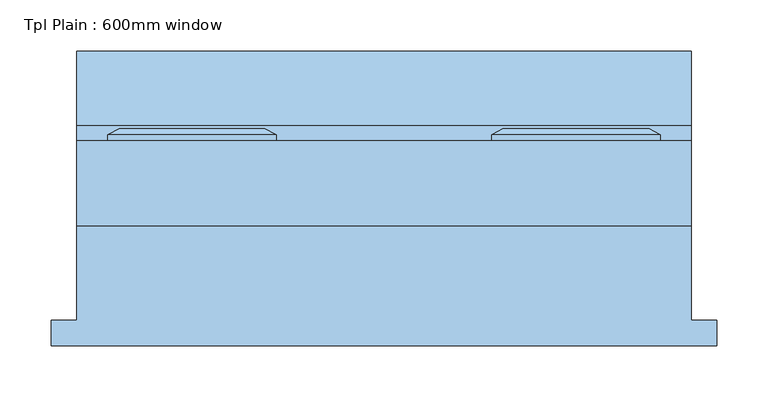
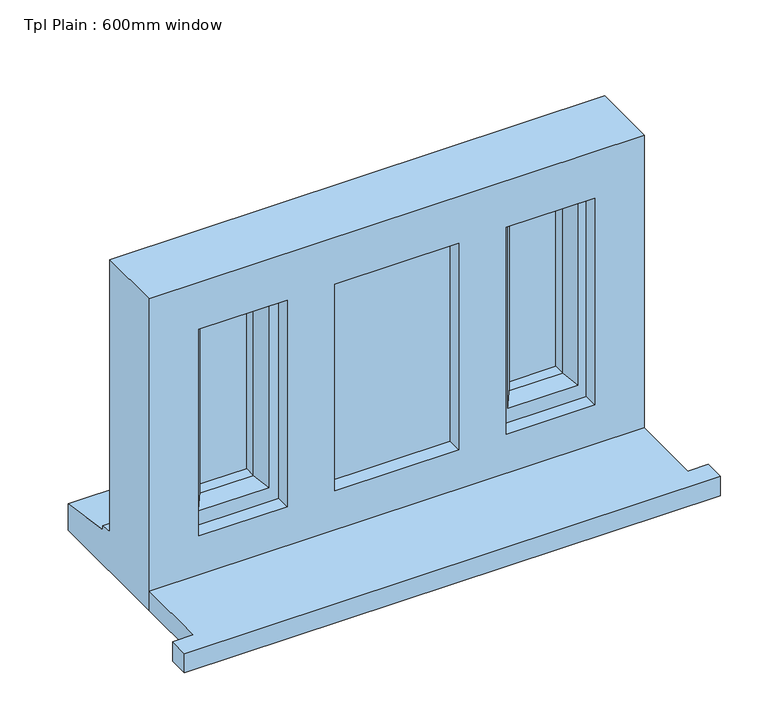
"""IFC4 building model written with IfcOpenShell, lengths in millimetres: window geometry, Tpl Plain : 600mm window."""

from ifc_helpers import new_model, si_unit, frame, origin, place, context, project, spatial, polyline, outline, extrude, faceted_brep, source, transform, mapped, element, save


def tpl_plain_600mm_window_e9a44080(model_context):
    return source(origin(), model_context, "Body", "SolidModel", [
        extrude(outline(polyline([(-700.0, -129.0434322), (-700.0, -104.0434322), (-675.0, -104.0434322), (-675.0, -12.0434322), (-75.0, -12.0434322), (-75.0, -104.0434322), (-50.0, -104.0434322), (-50.0, -129.0434322), (-700.0, -129.0434322)])), frame((0.0, 0.0, 2000.0), z_axis=(0.0, 0.0, 1.0), x_axis=(1.0, 0.0, 0.0)), (0.0, 0.0, 1.0), 25.0),
        faceted_brep([(-270.0, 70.9565678, 2370.0), (-270.0, 76.7300705, 2370.0), (-270.0, 76.7300705, 2053.0), (-270.0, 70.9565678, 2053.0), (-260.0, 5.9565678, 2360.0), (-260.0, 70.9565678, 2360.0), (-260.0, 70.9565678, 2063.0), (-260.0, 5.9565678, 2063.0), (-220.0, 20.4494677, 2320.0), (-230.1480377, 5.9565678, 2330.1480377), (-230.1480377, 5.9565678, 2092.8519623), (-220.0, 20.4494677, 2103.0), (-220.0, 34.9565678, 2320.0), (-220.0, 34.9565678, 2103.0), (-230.0, 58.9565678, 2330.0), (-230.0, 34.9565678, 2330.0), (-230.0, 34.9565678, 2093.0), (-230.0, 58.9565678, 2093.0), (-220.0, 76.7300705, 2320.0), (-220.0, 58.9565678, 2320.0), (-220.0, 58.9565678, 2103.0), (-220.0, 76.7300705, 2103.0), (-237.4457548, 82.5035732, 2337.4457548), (-237.4457548, 82.5035732, 2085.5542452), (-259.2153903, 82.5035732, 2359.2153903), (-259.2153903, 82.5035732, 2063.7846097), (-105.0, 76.7300705, 2053.0), (-105.0, 70.9565678, 2053.0), (-115.0, 70.9565678, 2063.0), (-115.0, 5.9565678, 2063.0), (-144.8519623, 5.9565678, 2092.8519623), (-155.0, 20.4494677, 2103.0), (-155.0, 34.9565678, 2103.0), (-145.0, 34.9565678, 2093.0), (-145.0, 58.9565678, 2093.0), (-155.0, 58.9565678, 2103.0), (-155.0, 76.7300705, 2103.0), (-137.5542452, 82.5035732, 2085.5542452), (-115.7846097, 82.5035732, 2063.7846097), (-105.0, 76.7300705, 2370.0), (-105.0, 70.9565678, 2370.0), (-115.0, 70.9565678, 2360.0), (-115.0, 5.9565678, 2360.0), (-144.8519623, 5.9565678, 2330.1480377), (-155.0, 20.4494677, 2320.0), (-155.0, 34.9565678, 2320.0), (-145.0, 34.9565678, 2330.0), (-145.0, 58.9565678, 2330.0), (-155.0, 58.9565678, 2320.0), (-155.0, 76.7300705, 2320.0), (-137.5542452, 82.5035732, 2337.4457548), (-115.7846097, 82.5035732, 2359.2153903)], [[[0, 1, 2, 3]], [[4, 5, 6, 7]], [[8, 9, 10, 11]], [[12, 8, 11, 13]], [[14, 15, 16, 17]], [[18, 19, 20, 21]], [[22, 18, 21, 23]], [[1, 24, 25, 2]], [[3, 2, 26, 27]], [[7, 6, 28, 29]], [[11, 10, 30, 31]], [[13, 11, 31, 32]], [[17, 16, 33, 34]], [[21, 20, 35, 36]], [[23, 21, 36, 37]], [[2, 25, 38, 26]], [[27, 26, 39, 40]], [[29, 28, 41, 42]], [[31, 30, 43, 44]], [[32, 31, 44, 45]], [[34, 33, 46, 47]], [[36, 35, 48, 49]], [[37, 36, 49, 50]], [[26, 38, 51, 39]], [[40, 39, 1, 0]], [[3, 27, 40, 0], [5, 41, 28, 6]], [[42, 41, 5, 4]], [[7, 29, 42, 4], [9, 43, 30, 10]], [[44, 43, 9, 8]], [[45, 44, 8, 12]], [[15, 46, 33, 16], [13, 32, 45, 12]], [[47, 46, 15, 14]], [[17, 34, 47, 14], [19, 48, 35, 20]], [[49, 48, 19, 18]], [[50, 49, 18, 22]], [[24, 51, 38, 25], [23, 37, 50, 22]], [[39, 51, 24, 1]]]),
        faceted_brep([(-480.0, 70.9565678, 2370.0), (-480.0, 76.7300705, 2370.0), (-645.0, 76.7300705, 2370.0), (-645.0, 70.9565678, 2370.0), (-490.0, 5.9565678, 2360.0), (-490.0, 70.9565678, 2360.0), (-635.0, 70.9565678, 2360.0), (-635.0, 5.9565678, 2360.0), (-530.0, 20.4494677, 2320.0), (-519.8519623, 5.9565678, 2330.1480377), (-605.1480377, 5.9565678, 2330.1480377), (-595.0, 20.4494677, 2320.0), (-530.0, 34.9565678, 2320.0), (-595.0, 34.9565678, 2320.0), (-520.0, 58.9565678, 2330.0), (-520.0, 34.9565678, 2330.0), (-605.0, 34.9565678, 2330.0), (-605.0, 58.9565678, 2330.0), (-530.0, 76.7300705, 2320.0), (-530.0, 58.9565678, 2320.0), (-595.0, 58.9565678, 2320.0), (-595.0, 76.7300705, 2320.0), (-511.1854344, 82.5035732, 2338.8145656), (-613.8145656, 82.5035732, 2338.8145656), (-491.6307806, 82.5035732, 2358.3692194), (-633.3692194, 82.5035732, 2358.3692194), (-645.0, 76.7300705, 2053.0), (-645.0, 70.9565678, 2053.0), (-635.0, 70.9565678, 2063.0), (-635.0, 5.9565678, 2063.0), (-605.1480377, 5.9565678, 2092.8519623), (-595.0, 20.4494677, 2103.0), (-595.0, 34.9565678, 2103.0), (-605.0, 34.9565678, 2093.0), (-605.0, 58.9565678, 2093.0), (-595.0, 58.9565678, 2103.0), (-595.0, 76.7300705, 2103.0), (-613.8145656, 82.5035732, 2084.1854344), (-633.3692194, 82.5035732, 2064.6307806), (-480.0, 76.7300705, 2053.0), (-480.0, 70.9565678, 2053.0), (-490.0, 70.9565678, 2063.0), (-490.0, 5.9565678, 2063.0), (-519.8519623, 5.9565678, 2092.8519623), (-530.0, 20.4494677, 2103.0), (-530.0, 34.9565678, 2103.0), (-520.0, 34.9565678, 2093.0), (-520.0, 58.9565678, 2093.0), (-530.0, 58.9565678, 2103.0), (-530.0, 76.7300705, 2103.0), (-511.1854344, 82.5035732, 2084.1854344), (-491.6307806, 82.5035732, 2064.6307806)], [[[0, 1, 2, 3]], [[4, 5, 6, 7]], [[8, 9, 10, 11]], [[12, 8, 11, 13]], [[14, 15, 16, 17]], [[18, 19, 20, 21]], [[22, 18, 21, 23]], [[1, 24, 25, 2]], [[3, 2, 26, 27]], [[7, 6, 28, 29]], [[11, 10, 30, 31]], [[13, 11, 31, 32]], [[17, 16, 33, 34]], [[21, 20, 35, 36]], [[23, 21, 36, 37]], [[2, 25, 38, 26]], [[27, 26, 39, 40]], [[0, 3, 27, 40], [41, 28, 6, 5]], [[29, 28, 41, 42]], [[4, 7, 29, 42], [43, 30, 10, 9]], [[31, 30, 43, 44]], [[32, 31, 44, 45]], [[46, 33, 16, 15], [12, 13, 32, 45]], [[34, 33, 46, 47]], [[14, 17, 34, 47], [48, 35, 20, 19]], [[36, 35, 48, 49]], [[37, 36, 49, 50]], [[51, 38, 25, 24], [22, 23, 37, 50]], [[26, 38, 51, 39]], [[40, 39, 1, 0]], [[42, 41, 5, 4]], [[44, 43, 9, 8]], [[45, 44, 8, 12]], [[47, 46, 15, 14]], [[49, 48, 19, 18]], [[50, 49, 18, 22]], [[39, 51, 24, 1]]]),
        faceted_brep([(-75.0, -12.0434322, 2400.0), (-675.0, -12.0434322, 2400.0), (-675.0, -12.0434322, 2000.0), (-75.0, -12.0434322, 2000.0), (-135.0, -12.0434322, 2340.0), (-135.0, -12.0434322, 2075.0), (-242.0, -12.0434322, 2075.0), (-242.0, -12.0434322, 2340.0), (-300.0, -12.0434322, 2340.0), (-300.0, -12.0434322, 2075.0), (-450.0, -12.0434322, 2075.0), (-450.0, -12.0434322, 2340.0), (-508.0, -12.0434322, 2340.0), (-508.0, -12.0434322, 2075.0), (-615.0, -12.0434322, 2075.0), (-615.0, -12.0434322, 2340.0), (-675.0, 70.9565678, 2400.0), (-675.0, 70.9565678, 2051.0), (-675.0, 85.9565678, 2049.68767), (-675.0, 85.9565678, 2044.7449676), (-675.0, 158.4565678, 2033.8088847), (-675.0, 158.4565678, 2000.0), (-75.0, 70.9565678, 2400.0), (-75.0, 70.9565678, 2051.0), (-635.0, 70.9565678, 2360.0), (-635.0, 70.9565678, 2063.0), (-490.0, 70.9565678, 2063.0), (-490.0, 70.9565678, 2360.0), (-450.0, 70.9565678, 2360.0), (-450.0, 70.9565678, 2063.0), (-300.0, 70.9565678, 2063.0), (-300.0, 70.9565678, 2360.0), (-260.0, 70.9565678, 2360.0), (-260.0, 70.9565678, 2063.0), (-115.0, 70.9565678, 2063.0), (-115.0, 70.9565678, 2360.0), (-635.0, 5.9565678, 2360.0), (-635.0, 5.9565678, 2063.0), (-460.0, 5.9565678, 2360.0), (-290.0, 5.9565678, 2360.0), (-290.0, 5.9565678, 2063.0), (-460.0, 5.9565678, 2063.0), (-300.0, 5.9565678, 2340.0), (-450.0, 5.9565678, 2340.0), (-450.0, 5.9565678, 2075.0), (-300.0, 5.9565678, 2075.0), (-260.0, 5.9565678, 2360.0), (-115.0, 5.9565678, 2360.0), (-115.0, 5.9565678, 2063.0), (-260.0, 5.9565678, 2063.0), (-135.0, 5.9565678, 2340.0), (-242.0, 5.9565678, 2340.0), (-242.0, 5.9565678, 2075.0), (-135.0, 5.9565678, 2075.0), (-490.0, 5.9565678, 2360.0), (-490.0, 5.9565678, 2063.0), (-508.0, 5.9565678, 2340.0), (-615.0, 5.9565678, 2340.0), (-615.0, 5.9565678, 2075.0), (-508.0, 5.9565678, 2075.0), (-450.0, 29.9565678, 2360.0), (-300.0, 29.9565678, 2360.0), (-290.0, 29.9565678, 2360.0), (-460.0, 29.9565678, 2360.0), (-75.0, 158.4565678, 2000.0), (-75.0, 158.4565678, 2033.8088847), (-75.0, 85.9565678, 2044.7449676), (-75.0, 85.9565678, 2049.68767), (-450.0, 29.9565678, 2063.0), (-460.0, 29.9565678, 2063.0), (-290.0, 29.9565678, 2063.0), (-300.0, 29.9565678, 2063.0)], [[[0, 1, 2, 3], [4, 5, 6, 7], [8, 9, 10, 11], [12, 13, 14, 15]], [[2, 1, 16, 17, 18, 19, 20, 21]], [[17, 16, 22, 23], [24, 25, 26, 27], [28, 29, 30, 31], [32, 33, 34, 35]], [[25, 24, 36, 37]], [[38, 39, 40, 41], [42, 43, 44, 45]], [[46, 47, 48, 49], [50, 51, 52, 53]], [[36, 54, 55, 37], [56, 57, 58, 59]], [[57, 15, 14, 58]], [[1, 0, 22, 16]], [[36, 24, 27, 54]], [[35, 47, 46, 32]], [[60, 28, 31, 61, 62, 39, 38, 63]], [[15, 57, 56, 12]], [[50, 4, 7, 51]], [[11, 43, 42, 8]], [[23, 22, 0, 3, 64, 65, 66, 67]], [[35, 34, 48, 47]], [[4, 50, 53, 5]], [[43, 11, 10, 44]], [[12, 56, 59, 13]], [[27, 26, 55, 54]], [[29, 28, 60, 68]], [[68, 60, 63, 69]], [[69, 63, 38, 41]], [[62, 70, 40, 39]], [[70, 62, 61, 71]], [[71, 61, 31, 30]], [[33, 32, 46, 49]], [[51, 7, 6, 52]], [[8, 42, 45, 9]], [[64, 3, 2, 21]], [[65, 64, 21, 20]], [[66, 65, 20, 19]], [[67, 66, 19, 18]], [[23, 67, 18, 17]], [[26, 25, 37, 55]], [[34, 33, 49, 48]], [[41, 40, 70, 71, 30, 29, 68, 69]], [[6, 5, 53, 52]], [[45, 44, 10, 9]], [[59, 58, 14, 13]]]),
        extrude(outline(polyline([(-520.0, 34.9565678), (-605.0, 34.9565678), (-605.0, 58.9565678), (-520.0, 58.9565678), (-520.0, 34.9565678)])), frame((0.0, 0.0, 2093.0), z_axis=(0.0, 0.0, 1.0), x_axis=(1.0, 0.0, 0.0)), (0.0, 0.0, 1.0), 237.0),
        extrude(outline(polyline([(-460.0, 29.9565678), (-290.0, 29.9565678), (-290.0, 5.9565678), (-460.0, 5.9565678), (-460.0, 29.9565678)])), frame((0.0, 0.0, 2063.0), z_axis=(0.0, 0.0, 1.0), x_axis=(1.0, 0.0, 0.0)), (0.0, 0.0, 1.0), 297.0),
        extrude(outline(polyline([(-145.0, 34.9565678), (-230.0, 34.9565678), (-230.0, 58.9565678), (-145.0, 58.9565678), (-145.0, 34.9565678)])), frame((0.0, 0.0, 2093.0), z_axis=(0.0, 0.0, 1.0), x_axis=(1.0, 0.0, 0.0)), (0.0, 0.0, 1.0), 237.0),
    ])


if __name__ == "__main__":
    model = new_model("IFC4")
    model_context = context("Model", 3, world=origin())
    ifc_project = project(units=[si_unit("LENGTHUNIT", "METRE", prefix="MILLI")], contexts=[model_context])
    site = spatial("IfcSite", under=ifc_project)
    building = spatial("IfcBuilding", under=site)
    placement = place(None, origin())
    tpl_plain_600mm_window_shape = tpl_plain_600mm_window_e9a44080(model_context)
    element("IfcWindow", 1, ObjectType="Tpl Plain : 600mm window", at=placement, inside=building, context=model_context, shape_type="MappedRepresentation", body=[
        mapped(tpl_plain_600mm_window_shape, transform((0.0, 0.0, 0.0), x_axis=(1.0, 0.0, 0.0), y_axis=(0.0, 1.0, 0.0), z_axis=(0.0, 0.0, 1.0))),
    ])
    save(model, "model.ifc")

# Revit data of these elements
# Type "Tpl Plain : 600mm window"
#   Type Mark = "33"
#   Operation = "TriplePanelVertical"
#   Manufacturer = "Revit"
#   Keynote = "L10"
#   Analytic Construction = "<None>"
#   Wrap Layers (Ext) from Ext = 102.5 mm
#   Wrap Layers (Int) from Ext = 177.5 mm
#   Window Board Projection = 25 mm
#   Window Board Extension = 25 mm
#   Rough Width = 600 mm
#   Rough Height = 400 mm
#   Height = 400 mm
#   Width = 600 mm
#   Glazing Thickness = 24 mm
#   FrameOffset - External = 50 mm
#   Frame Depth = 65 mm
#   Default Head Height = 2400 mm
#   Cill Depth = 87.5 mm
#   Cavity Closer Width = 50 mm
#   Cavity Closer Offset from Ext = 102.5 mm
#   Cavity Closer Depth = 85 mm
#   Vis - Cavity Closers = yes
#   Define Thermal Properties by = 1
#   Material Trim = Window Frame
#   Material Glass = Glass
#   Material Frame = Window Frame
#   Wall Closure = (empty or 0)
# Element 1 (IfcWindow, "Tpl Plain : 600mm window")
#   Materials on its faces: "Window Frame", "Glass"
# Materials
#   "Window Frame": colour RGB 249 249 249, transparency 0, Keynote = "L10", Cost = 0
#   "Glass": class "Glass", colour RGB 0 128 192, transparency 0.9, Description = "Soda Lime Glass", Cost = 0
